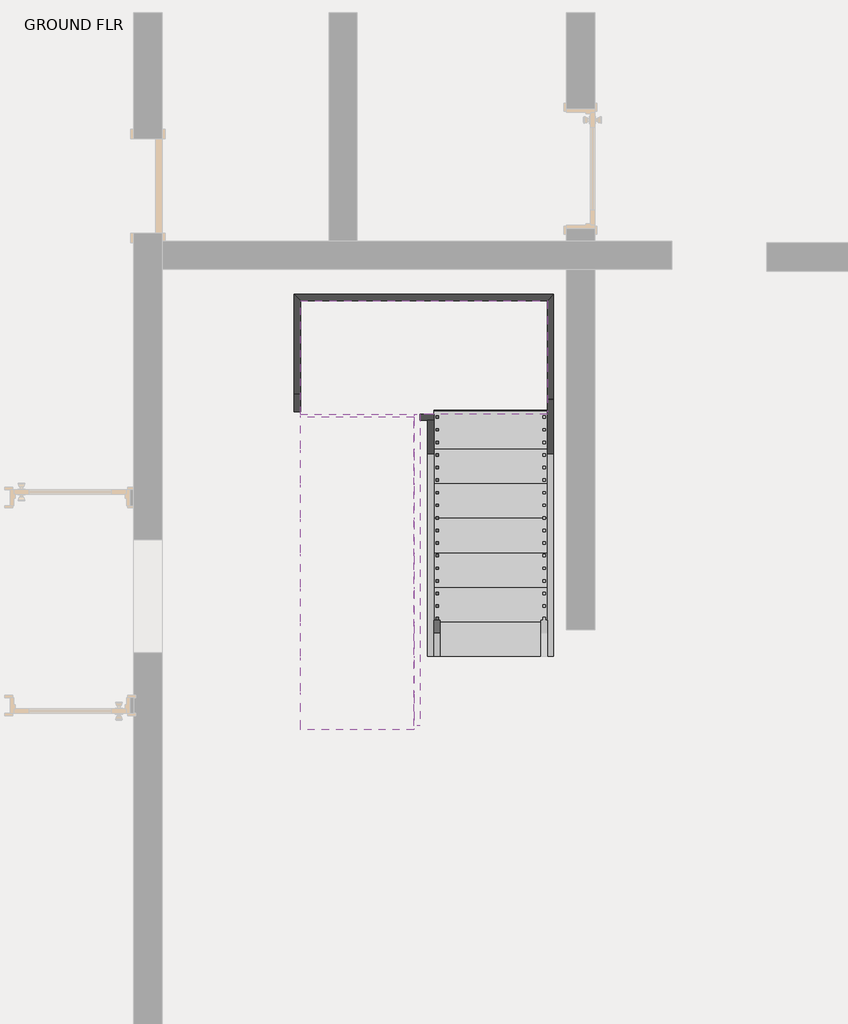
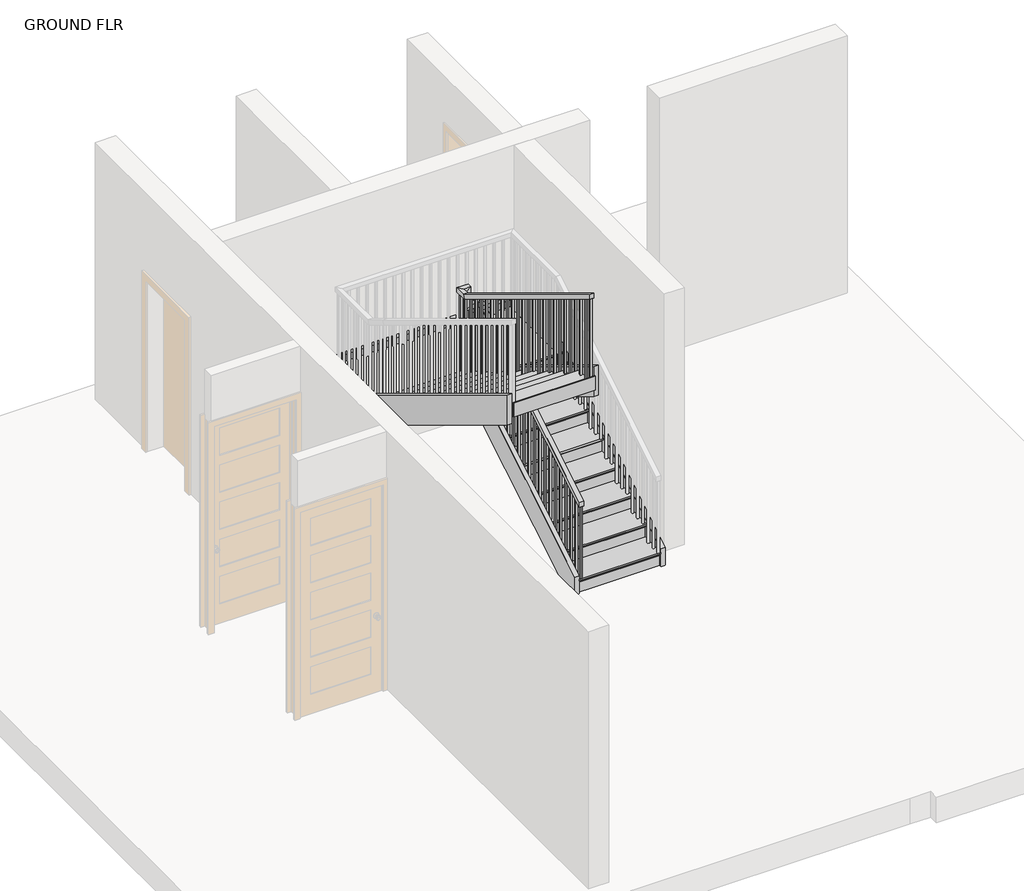
# One storey, part 3 of 3: 8 members, 2 stair flights, 1 railing, 1 slab.
"""IFC4 building model written with IfcOpenShell, lengths in millimetres."""

from ifc_helpers import new_model, si_unit, frame, origin, place, context, project, spatial, polyline, outline, extrude, faceted_brep, transform, mapped, element, save
from components import non_monolithic_landing_8dc99a10, stair_flight_27979845, stair_flight_611140c6

model = new_model("IFC4")

# Units and contexts
model_context = context("Model", 3, world=origin())
ifc_project = project(units=[si_unit("LENGTHUNIT", "METRE", prefix="MILLI")], contexts=[model_context])

# Site, building, storey
site = spatial("IfcSite", under=ifc_project)
building = spatial("IfcBuilding", under=site)
storey = spatial("IfcBuildingStorey", under=building, Name="GROUND FLR", Elevation=609.6)

# Members
placement = place(None, origin())
element("IfcMember", 1, ObjectType="Stringer - 2\" Width", at=placement, inside=storey, context=model_context, shape_type="SweptSolid", body=[
    extrude(outline(polyline([(-3250.5249317, 609.6), (-3250.5249317, 821.714512), (-1345.5249317, 1976.2599665), (-1345.5249317, 1619.851205), (-3012.4394199, 609.6), (-3250.5249317, 609.6)])), frame((-6345.6481169, 0.0, 0.0), z_axis=(1.0, 0.0, 0.0), x_axis=(0.0, 1.0, 0.0)), (0.0, 0.0, 1.0), 50.8),
])
element("IfcMember", 2, ObjectType="Stringer - 2\" Width", at=placement, inside=storey, context=model_context, shape_type="SweptSolid", body=[
    extrude(outline(polyline([(-3250.5249317, 609.6), (-3250.5249317, 821.714512), (-1239.5838764, 2040.4666667), (-1154.4294199, 1735.6666667), (-3012.4394199, 609.6), (-3250.5249317, 609.6)])), frame((-5380.4481169, 0.0, 0.0), z_axis=(1.0, 0.0, 0.0), x_axis=(0.0, 1.0, 0.0)), (0.0, 0.0, 1.0), 50.8),
])
element("IfcMember", 3, ObjectType="Stringer - 2\" Width", at=placement, inside=storey, context=model_context, shape_type="SweptSolid", body=[
    extrude(outline(polyline([(-1294.7249317, 2176.3811786), (-1294.7249317, 1819.9724171), (-3809.3249317, 3343.9724171), (-3809.3249317, 3700.3811786), (-1294.7249317, 2176.3811786)])), frame((-6457.6431792, 0.0, 0.0), z_axis=(1.0, 0.0, 0.0), x_axis=(0.0, 1.0, 0.0)), (0.0, 0.0, 1.0), 50.8),
])
element("IfcMember", 4, ObjectType="Stringer - 2\" Width", at=placement, inside=storey, context=model_context, shape_type="SweptSolid", body=[
    extrude(outline(polyline([(-1070.465987, 2040.4666667), (-1155.6204435, 1735.6666667), (-3809.3249317, 3343.9724171), (-3809.3249317, 3700.3811786), (-1070.465987, 2040.4666667)])), frame((-7422.8431792, 0.0, 0.0), z_axis=(1.0, 0.0, 0.0), x_axis=(0.0, 1.0, 0.0)), (0.0, 0.0, 1.0), 50.8),
])
element("IfcMember", 5, ObjectType="Stringer - 2\" Width", at=placement, inside=storey, context=model_context, shape_type="SweptSolid", body=[
    extrude(outline(polyline([(-6406.8431792, -1345.5249317), (-6406.8431792, -1294.7249317), (-6294.8481169, -1294.7249317), (-6294.8481169, -1345.5249317), (-6406.8431792, -1345.5249317)])), frame((0.0, 0.0, 1735.6666667), z_axis=(0.0, 0.0, 1.0), x_axis=(1.0, 0.0, 0.0)), (0.0, 0.0, 1.0), 304.8),
])
element("IfcMember", 6, ObjectType="Stringer - 2\" Width", at=placement, inside=storey, context=model_context, shape_type="Brep", body=[
    faceted_brep([(-5380.4481169, -1239.5838764, 2040.4666667), (-5329.6481169, -1239.5838764, 2040.4666667), (-5329.6481169, -329.5249317, 2040.4666667), (-5380.4481169, -380.3249317, 2040.4666667), (-5380.4481169, -1154.4294199, 1735.6666667), (-5380.4481169, -380.3249317, 1735.6666667), (-5329.6481169, -1154.4294199, 1735.6666667), (-5329.6481169, -329.5249317, 1735.6666667)], [[[0, 1, 2, 3]], [[4, 0, 3, 5]], [[6, 4, 5, 7]], [[1, 6, 7, 2]], [[1, 0, 4, 6]], [[2, 7, 5, 3]]]),
])
element("IfcMember", 7, ObjectType="Stringer - 2\" Width", at=placement, inside=storey, context=model_context, shape_type="SweptSolid", body=[
    extrude(outline(polyline([(-5329.6481169, -329.5249317), (-5380.4481169, -380.3249317), (-7372.0431792, -380.3249317), (-7422.8431792, -329.5249317), (-5329.6481169, -329.5249317)])), frame((0.0, 0.0, 1735.6666667), z_axis=(0.0, 0.0, 1.0), x_axis=(1.0, 0.0, 0.0)), (0.0, 0.0, 1.0), 304.8),
])
element("IfcMember", 8, ObjectType="Stringer - 2\" Width", at=placement, inside=storey, context=model_context, shape_type="Brep", body=[
    faceted_brep([(-7372.0431792, -380.3249317, 2040.4666667), (-7422.8431792, -329.5249317, 2040.4666667), (-7422.8431792, -1070.465987, 2040.4666667), (-7372.0431792, -1070.465987, 2040.4666667), (-7372.0431792, -380.3249317, 1735.6666667), (-7372.0431792, -1155.6204435, 1735.6666667), (-7422.8431792, -329.5249317, 1735.6666667), (-7422.8431792, -1155.6204435, 1735.6666667)], [[[0, 1, 2, 3]], [[4, 0, 3, 5]], [[6, 4, 5, 7]], [[1, 6, 7, 2]], [[1, 0, 4, 6]], [[2, 7, 5, 3]]]),
])

# Railing
element("IfcRailing", 9, ObjectType="Handrail - Rectangular", at=placement, inside=storey, context=model_context, shape_type="SolidModel", body=[
    faceted_brep([(-6294.8481169, -3250.5249317, 1693.3333333), (-6294.8481169, -3250.5249317, 1633.9318731), (-6244.0481169, -3250.5249317, 1633.9318731), (-6244.0481169, -3250.5249317, 1693.3333333), (-6294.8481169, -1370.9249317, 2832.4848485), (-6294.8481169, -1320.1249317, 2803.871267), (-6244.0481169, -1320.1249317, 2803.871267), (-6244.0481169, -1370.9249317, 2832.4848485), (-6294.8481169, -1370.9249317, 2878.6666667), (-6294.8481169, -1320.1249317, 2827.8666667), (-6244.0481169, -1320.1249317, 2827.8666667), (-6244.0481169, -1370.9249317, 2878.6666667), (-6294.8481169, -1294.7249317, 2878.6666667), (-6294.8481169, -1294.7249317, 2827.8666667), (-6244.0481169, -1243.9249317, 2827.8666667), (-6244.0481169, -1243.9249317, 2878.6666667), (-6371.0481169, -1294.7249317, 2878.6666667), (-6371.0481169, -1294.7249317, 2827.8666667), (-6371.0481169, -1243.9249317, 2827.8666667), (-6371.0481169, -1243.9249317, 2878.6666667), (-6381.4431792, -1294.7249317, 2878.6666667), (-6432.2431792, -1294.7249317, 2827.8666667), (-6432.2431792, -1243.9249317, 2827.8666667), (-6381.4431792, -1243.9249317, 2878.6666667), (-6381.4431792, -1294.7249317, 3094.1818182), (-6432.2431792, -1294.7249317, 3043.3818182), (-6432.2431792, -1243.9249317, 3043.3818182), (-6381.4431792, -1243.9249317, 3094.1818182), (-6457.6431792, -1294.7249317, 3094.1818182), (-6457.6431792, -1294.7249317, 3043.3818182), (-6508.4431792, -1243.9249317, 3043.3818182), (-6508.4431792, -1243.9249317, 3094.1818182), (-6457.6431792, -1370.9249317, 3094.1818182), (-6457.6431792, -1385.1173411, 3043.3818182), (-6508.4431792, -1385.1173411, 3043.3818182), (-6508.4431792, -1370.9249317, 3094.1818182), (-6457.6431792, -3809.3249317, 4572.0), (-6508.4431792, -3809.3249317, 4572.0), (-6508.4431792, -3809.3249317, 4512.5985397), (-6457.6431792, -3809.3249317, 4512.5985397)], [[[0, 1, 2, 3]], [[1, 0, 4, 5]], [[2, 1, 5, 6]], [[3, 2, 6, 7]], [[0, 3, 7, 4]], [[5, 4, 8, 9]], [[6, 5, 9, 10]], [[7, 6, 10, 11]], [[4, 7, 11, 8]], [[9, 8, 12, 13]], [[10, 9, 13, 14]], [[11, 10, 14, 15]], [[8, 11, 15, 12]], [[13, 12, 16, 17]], [[14, 13, 17, 18]], [[15, 14, 18, 19]], [[12, 15, 19, 16]], [[17, 16, 20, 21]], [[18, 17, 21, 22]], [[19, 18, 22, 23]], [[16, 19, 23, 20]], [[21, 20, 24, 25]], [[22, 21, 25, 26]], [[23, 22, 26, 27]], [[20, 23, 27, 24]], [[25, 24, 28, 29]], [[26, 25, 29, 30]], [[27, 26, 30, 31]], [[24, 27, 31, 28]], [[29, 28, 32, 33]], [[30, 29, 33, 34]], [[31, 30, 34, 35]], [[28, 31, 35, 32]], [[36, 37, 38, 39]], [[33, 32, 36, 39]], [[34, 33, 39, 38]], [[35, 34, 38, 37]], [[32, 35, 37, 36]]]),
    extrude(outline(polyline([(-3698.1999317, 4445.2500549), (-3698.1999317, 3488.2666667), (-3717.2499317, 3488.2666667), (-3717.2499317, 4456.7955094), (-3698.1999317, 4445.2500549)])), frame((-6492.5681792, 0.0, 0.0), z_axis=(1.0, 0.0, 0.0), x_axis=(0.0, 1.0, 0.0)), (0.0, 0.0, 1.0), 19.05),
    extrude(outline(polyline([(-3596.5999317, 4383.6742973), (-3596.5999317, 3488.2666667), (-3615.6499317, 3488.2666667), (-3615.6499317, 4395.2197519), (-3596.5999317, 4383.6742973)])), frame((-6492.5681792, 0.0, 0.0), z_axis=(1.0, 0.0, 0.0), x_axis=(0.0, 1.0, 0.0)), (0.0, 0.0, 1.0), 19.05),
    extrude(outline(polyline([(-3494.9999317, 4322.0985397), (-3494.9999317, 3318.9333333), (-3514.0499317, 3318.9333333), (-3514.0499317, 4333.6439943), (-3494.9999317, 4322.0985397)])), frame((-6492.5681792, 0.0, 0.0), z_axis=(1.0, 0.0, 0.0), x_axis=(0.0, 1.0, 0.0)), (0.0, 0.0, 1.0), 19.05),
    extrude(outline(polyline([(-3393.3999317, 4260.5227822), (-3393.3999317, 3318.9333333), (-3412.4499317, 3318.9333333), (-3412.4499317, 4272.0682367), (-3393.3999317, 4260.5227822)])), frame((-6492.5681792, 0.0, 0.0), z_axis=(1.0, 0.0, 0.0), x_axis=(0.0, 1.0, 0.0)), (0.0, 0.0, 1.0), 19.05),
    extrude(outline(polyline([(-3291.7999317, 4198.9470246), (-3291.7999317, 3318.9333333), (-3310.8499317, 3318.9333333), (-3310.8499317, 4210.4924791), (-3291.7999317, 4198.9470246)])), frame((-6492.5681792, 0.0, 0.0), z_axis=(1.0, 0.0, 0.0), x_axis=(0.0, 1.0, 0.0)), (0.0, 0.0, 1.0), 19.05),
    extrude(outline(polyline([(-3190.1999317, 4137.371267), (-3190.1999317, 3149.6), (-3209.2499317, 3149.6), (-3209.2499317, 4148.9167216), (-3190.1999317, 4137.371267)])), frame((-6492.5681792, 0.0, 0.0), z_axis=(1.0, 0.0, 0.0), x_axis=(0.0, 1.0, 0.0)), (0.0, 0.0, 1.0), 19.05),
    extrude(outline(polyline([(-3088.5999317, 4075.7955094), (-3088.5999317, 3149.6), (-3107.6499317, 3149.6), (-3107.6499317, 4087.340964), (-3088.5999317, 4075.7955094)])), frame((-6492.5681792, 0.0, 0.0), z_axis=(1.0, 0.0, 0.0), x_axis=(0.0, 1.0, 0.0)), (0.0, 0.0, 1.0), 19.05),
    extrude(outline(polyline([(-2986.9999317, 4014.2197519), (-2986.9999317, 3149.6), (-3006.0499317, 3149.6), (-3006.0499317, 4025.7652064), (-2986.9999317, 4014.2197519)])), frame((-6492.5681792, 0.0, 0.0), z_axis=(1.0, 0.0, 0.0), x_axis=(0.0, 1.0, 0.0)), (0.0, 0.0, 1.0), 19.05),
    extrude(outline(polyline([(-2885.3999317, 3952.6439943), (-2885.3999317, 2980.2666667), (-2904.4499317, 2980.2666667), (-2904.4499317, 3964.1894488), (-2885.3999317, 3952.6439943)])), frame((-6492.5681792, 0.0, 0.0), z_axis=(1.0, 0.0, 0.0), x_axis=(0.0, 1.0, 0.0)), (0.0, 0.0, 1.0), 19.05),
    extrude(outline(polyline([(-2783.7999317, 3891.0682367), (-2783.7999317, 2980.2666667), (-2802.8499317, 2980.2666667), (-2802.8499317, 3902.6136913), (-2783.7999317, 3891.0682367)])), frame((-6492.5681792, 0.0, 0.0), z_axis=(1.0, 0.0, 0.0), x_axis=(0.0, 1.0, 0.0)), (0.0, 0.0, 1.0), 19.05),
    extrude(outline(polyline([(-2682.1999317, 3829.4924791), (-2682.1999317, 2980.2666667), (-2701.2499317, 2980.2666667), (-2701.2499317, 3841.0379337), (-2682.1999317, 3829.4924791)])), frame((-6492.5681792, 0.0, 0.0), z_axis=(1.0, 0.0, 0.0), x_axis=(0.0, 1.0, 0.0)), (0.0, 0.0, 1.0), 19.05),
    extrude(outline(polyline([(-2580.5999317, 3767.9167216), (-2580.5999317, 2810.9333333), (-2599.6499317, 2810.9333333), (-2599.6499317, 3779.4621761), (-2580.5999317, 3767.9167216)])), frame((-6492.5681792, 0.0, 0.0), z_axis=(1.0, 0.0, 0.0), x_axis=(0.0, 1.0, 0.0)), (0.0, 0.0, 1.0), 19.05),
    extrude(outline(polyline([(-2478.9999317, 3706.340964), (-2478.9999317, 2810.9333333), (-2498.0499317, 2810.9333333), (-2498.0499317, 3717.8864185), (-2478.9999317, 3706.340964)])), frame((-6492.5681792, 0.0, 0.0), z_axis=(1.0, 0.0, 0.0), x_axis=(0.0, 1.0, 0.0)), (0.0, 0.0, 1.0), 19.05),
    extrude(outline(polyline([(-2377.3999317, 3644.7652064), (-2377.3999317, 2641.6), (-2396.4499317, 2641.6), (-2396.4499317, 3656.310661), (-2377.3999317, 3644.7652064)])), frame((-6492.5681792, 0.0, 0.0), z_axis=(1.0, 0.0, 0.0), x_axis=(0.0, 1.0, 0.0)), (0.0, 0.0, 1.0), 19.05),
    extrude(outline(polyline([(-2275.7999317, 3583.1894488), (-2275.7999317, 2641.6), (-2294.8499317, 2641.6), (-2294.8499317, 3594.7349034), (-2275.7999317, 3583.1894488)])), frame((-6492.5681792, 0.0, 0.0), z_axis=(1.0, 0.0, 0.0), x_axis=(0.0, 1.0, 0.0)), (0.0, 0.0, 1.0), 19.05),
    extrude(outline(polyline([(-2174.1999317, 3521.6136913), (-2174.1999317, 2641.6), (-2193.2499317, 2641.6), (-2193.2499317, 3533.1591458), (-2174.1999317, 3521.6136913)])), frame((-6492.5681792, 0.0, 0.0), z_axis=(1.0, 0.0, 0.0), x_axis=(0.0, 1.0, 0.0)), (0.0, 0.0, 1.0), 19.05),
    extrude(outline(polyline([(-2072.5999317, 3460.0379337), (-2072.5999317, 2472.2666667), (-2091.6499317, 2472.2666667), (-2091.6499317, 3471.5833882), (-2072.5999317, 3460.0379337)])), frame((-6492.5681792, 0.0, 0.0), z_axis=(1.0, 0.0, 0.0), x_axis=(0.0, 1.0, 0.0)), (0.0, 0.0, 1.0), 19.05),
    extrude(outline(polyline([(-1970.9999317, 3398.4621761), (-1970.9999317, 2472.2666667), (-1990.0499317, 2472.2666667), (-1990.0499317, 3410.0076307), (-1970.9999317, 3398.4621761)])), frame((-6492.5681792, 0.0, 0.0), z_axis=(1.0, 0.0, 0.0), x_axis=(0.0, 1.0, 0.0)), (0.0, 0.0, 1.0), 19.05),
    extrude(outline(polyline([(-1869.3999317, 3336.8864185), (-1869.3999317, 2472.2666667), (-1888.4499317, 2472.2666667), (-1888.4499317, 3348.4318731), (-1869.3999317, 3336.8864185)])), frame((-6492.5681792, 0.0, 0.0), z_axis=(1.0, 0.0, 0.0), x_axis=(0.0, 1.0, 0.0)), (0.0, 0.0, 1.0), 19.05),
    extrude(outline(polyline([(-1767.7999317, 3275.310661), (-1767.7999317, 2302.9333333), (-1786.8499317, 2302.9333333), (-1786.8499317, 3286.8561155), (-1767.7999317, 3275.310661)])), frame((-6492.5681792, 0.0, 0.0), z_axis=(1.0, 0.0, 0.0), x_axis=(0.0, 1.0, 0.0)), (0.0, 0.0, 1.0), 19.05),
    extrude(outline(polyline([(-1666.1999317, 3213.7349034), (-1666.1999317, 2302.9333333), (-1685.2499317, 2302.9333333), (-1685.2499317, 3225.2803579), (-1666.1999317, 3213.7349034)])), frame((-6492.5681792, 0.0, 0.0), z_axis=(1.0, 0.0, 0.0), x_axis=(0.0, 1.0, 0.0)), (0.0, 0.0, 1.0), 19.05),
    extrude(outline(polyline([(-1564.5999317, 3152.1591458), (-1564.5999317, 2302.9333333), (-1583.6499317, 2302.9333333), (-1583.6499317, 3163.7046004), (-1564.5999317, 3152.1591458)])), frame((-6492.5681792, 0.0, 0.0), z_axis=(1.0, 0.0, 0.0), x_axis=(0.0, 1.0, 0.0)), (0.0, 0.0, 1.0), 19.05),
    extrude(outline(polyline([(-1462.9999317, 3090.5833882), (-1462.9999317, 2133.6), (-1482.0499317, 2133.6), (-1482.0499317, 3102.1288428), (-1462.9999317, 3090.5833882)])), frame((-6492.5681792, 0.0, 0.0), z_axis=(1.0, 0.0, 0.0), x_axis=(0.0, 1.0, 0.0)), (0.0, 0.0, 1.0), 19.05),
    extrude(outline(polyline([(-1361.3999317, 3029.0076307), (-1361.3999317, 2133.6), (-1380.4499317, 2133.6), (-1380.4499317, 3040.5530852), (-1361.3999317, 3029.0076307)])), frame((-6492.5681792, 0.0, 0.0), z_axis=(1.0, 0.0, 0.0), x_axis=(0.0, 1.0, 0.0)), (0.0, 0.0, 1.0), 19.05),
    extrude(outline(polyline([(-6463.1231169, -1278.8499317), (-6482.1731169, -1278.8499317), (-6482.1731169, -1259.7999317), (-6463.1231169, -1259.7999317), (-6463.1231169, -1278.8499317)])), frame((0.0, 0.0, 1964.2666667), z_axis=(0.0, 0.0, 1.0), x_axis=(1.0, 0.0, 0.0)), (0.0, 0.0, 1.0), 1079.1151515),
    extrude(outline(polyline([(-6361.5231169, -1278.8499317), (-6380.5731169, -1278.8499317), (-6380.5731169, -1259.7999317), (-6361.5231169, -1259.7999317), (-6361.5231169, -1278.8499317)])), frame((0.0, 0.0, 1964.2666667), z_axis=(0.0, 0.0, 1.0), x_axis=(1.0, 0.0, 0.0)), (0.0, 0.0, 1.0), 863.6),
    extrude(outline(polyline([(-6278.9731169, -1329.6499317), (-6278.9731169, -1310.5999317), (-6259.9231169, -1310.5999317), (-6259.9231169, -1329.6499317), (-6278.9731169, -1329.6499317)])), frame((0.0, 0.0, 1794.9333333), z_axis=(0.0, 0.0, 1.0), x_axis=(1.0, 0.0, 0.0)), (0.0, 0.0, 1.0), 1032.9333333),
    extrude(outline(polyline([(-1412.1999317, 2748.0682367), (-1412.1999317, 1794.9333333), (-1431.2499317, 1794.9333333), (-1431.2499317, 2736.5227822), (-1412.1999317, 2748.0682367)])), frame((-6278.9731169, 0.0, 0.0), z_axis=(1.0, 0.0, 0.0), x_axis=(0.0, 1.0, 0.0)), (0.0, 0.0, 1.0), 19.05),
    extrude(outline(polyline([(-1513.7999317, 2686.4924791), (-1513.7999317, 1794.9333333), (-1532.8499317, 1794.9333333), (-1532.8499317, 2674.9470246), (-1513.7999317, 2686.4924791)])), frame((-6278.9731169, 0.0, 0.0), z_axis=(1.0, 0.0, 0.0), x_axis=(0.0, 1.0, 0.0)), (0.0, 0.0, 1.0), 19.05),
    extrude(outline(polyline([(-1615.3999317, 2624.9167216), (-1615.3999317, 1625.6), (-1634.4499317, 1625.6), (-1634.4499317, 2613.371267), (-1615.3999317, 2624.9167216)])), frame((-6278.9731169, 0.0, 0.0), z_axis=(1.0, 0.0, 0.0), x_axis=(0.0, 1.0, 0.0)), (0.0, 0.0, 1.0), 19.05),
    extrude(outline(polyline([(-1716.9999317, 2563.340964), (-1716.9999317, 1625.6), (-1736.0499317, 1625.6), (-1736.0499317, 2551.7955094), (-1716.9999317, 2563.340964)])), frame((-6278.9731169, 0.0, 0.0), z_axis=(1.0, 0.0, 0.0), x_axis=(0.0, 1.0, 0.0)), (0.0, 0.0, 1.0), 19.05),
    extrude(outline(polyline([(-1818.5999317, 2501.7652064), (-1818.5999317, 1625.6), (-1837.6499317, 1625.6), (-1837.6499317, 2490.2197519), (-1818.5999317, 2501.7652064)])), frame((-6278.9731169, 0.0, 0.0), z_axis=(1.0, 0.0, 0.0), x_axis=(0.0, 1.0, 0.0)), (0.0, 0.0, 1.0), 19.05),
    extrude(outline(polyline([(-1920.1999317, 2440.1894488), (-1920.1999317, 1456.2666667), (-1939.2499317, 1456.2666667), (-1939.2499317, 2428.6439943), (-1920.1999317, 2440.1894488)])), frame((-6278.9731169, 0.0, 0.0), z_axis=(1.0, 0.0, 0.0), x_axis=(0.0, 1.0, 0.0)), (0.0, 0.0, 1.0), 19.05),
    extrude(outline(polyline([(-2021.7999317, 2378.6136913), (-2021.7999317, 1456.2666667), (-2040.8499317, 1456.2666667), (-2040.8499317, 2367.0682367), (-2021.7999317, 2378.6136913)])), frame((-6278.9731169, 0.0, 0.0), z_axis=(1.0, 0.0, 0.0), x_axis=(0.0, 1.0, 0.0)), (0.0, 0.0, 1.0), 19.05),
    extrude(outline(polyline([(-2123.3999317, 2317.0379337), (-2123.3999317, 1456.2666667), (-2142.4499317, 1456.2666667), (-2142.4499317, 2305.4924791), (-2123.3999317, 2317.0379337)])), frame((-6278.9731169, 0.0, 0.0), z_axis=(1.0, 0.0, 0.0), x_axis=(0.0, 1.0, 0.0)), (0.0, 0.0, 1.0), 19.05),
    extrude(outline(polyline([(-2224.9999317, 2255.4621761), (-2224.9999317, 1286.9333333), (-2244.0499317, 1286.9333333), (-2244.0499317, 2243.9167216), (-2224.9999317, 2255.4621761)])), frame((-6278.9731169, 0.0, 0.0), z_axis=(1.0, 0.0, 0.0), x_axis=(0.0, 1.0, 0.0)), (0.0, 0.0, 1.0), 19.05),
    extrude(outline(polyline([(-2326.5999317, 2193.8864185), (-2326.5999317, 1286.9333333), (-2345.6499317, 1286.9333333), (-2345.6499317, 2182.340964), (-2326.5999317, 2193.8864185)])), frame((-6278.9731169, 0.0, 0.0), z_axis=(1.0, 0.0, 0.0), x_axis=(0.0, 1.0, 0.0)), (0.0, 0.0, 1.0), 19.05),
    extrude(outline(polyline([(-2428.1999317, 2132.310661), (-2428.1999317, 1117.6), (-2447.2499317, 1117.6), (-2447.2499317, 2120.7652064), (-2428.1999317, 2132.310661)])), frame((-6278.9731169, 0.0, 0.0), z_axis=(1.0, 0.0, 0.0), x_axis=(0.0, 1.0, 0.0)), (0.0, 0.0, 1.0), 19.05),
    extrude(outline(polyline([(-2529.7999317, 2070.7349034), (-2529.7999317, 1117.6), (-2548.8499317, 1117.6), (-2548.8499317, 2059.1894488), (-2529.7999317, 2070.7349034)])), frame((-6278.9731169, 0.0, 0.0), z_axis=(1.0, 0.0, 0.0), x_axis=(0.0, 1.0, 0.0)), (0.0, 0.0, 1.0), 19.05),
    extrude(outline(polyline([(-2631.3999317, 2009.1591458), (-2631.3999317, 1117.6), (-2650.4499317, 1117.6), (-2650.4499317, 1997.6136913), (-2631.3999317, 2009.1591458)])), frame((-6278.9731169, 0.0, 0.0), z_axis=(1.0, 0.0, 0.0), x_axis=(0.0, 1.0, 0.0)), (0.0, 0.0, 1.0), 19.05),
    extrude(outline(polyline([(-2732.9999317, 1947.5833882), (-2732.9999317, 948.2666667), (-2752.0499317, 948.2666667), (-2752.0499317, 1936.0379337), (-2732.9999317, 1947.5833882)])), frame((-6278.9731169, 0.0, 0.0), z_axis=(1.0, 0.0, 0.0), x_axis=(0.0, 1.0, 0.0)), (0.0, 0.0, 1.0), 19.05),
    extrude(outline(polyline([(-2834.5999317, 1886.0076307), (-2834.5999317, 948.2666667), (-2853.6499317, 948.2666667), (-2853.6499317, 1874.4621761), (-2834.5999317, 1886.0076307)])), frame((-6278.9731169, 0.0, 0.0), z_axis=(1.0, 0.0, 0.0), x_axis=(0.0, 1.0, 0.0)), (0.0, 0.0, 1.0), 19.05),
    extrude(outline(polyline([(-2936.1999317, 1824.4318731), (-2936.1999317, 948.2666667), (-2955.2499317, 948.2666667), (-2955.2499317, 1812.8864185), (-2936.1999317, 1824.4318731)])), frame((-6278.9731169, 0.0, 0.0), z_axis=(1.0, 0.0, 0.0), x_axis=(0.0, 1.0, 0.0)), (0.0, 0.0, 1.0), 19.05),
    extrude(outline(polyline([(-3037.7999317, 1762.8561155), (-3037.7999317, 778.9333333), (-3056.8499317, 778.9333333), (-3056.8499317, 1751.310661), (-3037.7999317, 1762.8561155)])), frame((-6278.9731169, 0.0, 0.0), z_axis=(1.0, 0.0, 0.0), x_axis=(0.0, 1.0, 0.0)), (0.0, 0.0, 1.0), 19.05),
    extrude(outline(polyline([(-3139.3999317, 1701.2803579), (-3139.3999317, 778.9333333), (-3158.4499317, 778.9333333), (-3158.4499317, 1689.7349034), (-3139.3999317, 1701.2803579)])), frame((-6278.9731169, 0.0, 0.0), z_axis=(1.0, 0.0, 0.0), x_axis=(0.0, 1.0, 0.0)), (0.0, 0.0, 1.0), 19.05),
    extrude(outline(polyline([(-6473.5181792, -1278.8499317), (-6492.5681792, -1278.8499317), (-6492.5681792, -1259.7999317), (-6473.5181792, -1259.7999317), (-6473.5181792, -1278.8499317)])), frame((0.0, 0.0, 1964.2666667), z_axis=(0.0, 0.0, 1.0), x_axis=(1.0, 0.0, 0.0)), (0.0, 0.0, 1.0), 1079.1151515),
    extrude(outline(polyline([(-6278.9731169, -1278.8499317), (-6278.9731169, -1259.7999317), (-6259.9231169, -1259.7999317), (-6259.9231169, -1278.8499317), (-6278.9731169, -1278.8499317)])), frame((0.0, 0.0, 1964.2666667), z_axis=(0.0, 0.0, 1.0), x_axis=(1.0, 0.0, 0.0)), (0.0, 0.0, 1.0), 863.6),
    extrude(outline(polyline([(-3790.2749317, 4501.0530852), (-3790.2749317, 3488.2666667), (-3809.3249317, 3488.2666667), (-3809.3249317, 4512.5985397), (-3790.2749317, 4501.0530852)])), frame((-6492.5681792, 0.0, 0.0), z_axis=(1.0, 0.0, 0.0), x_axis=(0.0, 1.0, 0.0)), (0.0, 0.0, 1.0), 19.05),
    extrude(outline(polyline([(-3231.4749317, 1645.4773276), (-3231.4749317, 778.9333333), (-3250.5249317, 778.9333333), (-3250.5249317, 1633.9318731), (-3231.4749317, 1645.4773276)])), frame((-6278.9731169, 0.0, 0.0), z_axis=(1.0, 0.0, 0.0), x_axis=(0.0, 1.0, 0.0)), (0.0, 0.0, 1.0), 19.05),
])

# Slab
non_monolithic_landing_shape = non_monolithic_landing_8dc99a10(model_context)
element("IfcSlab", 10, ObjectType="Non-Monolithic Landing", at=placement, inside=storey, context=model_context, shape_type="MappedRepresentation", body=[
    mapped(non_monolithic_landing_shape, transform((0.0, 0.0, 0.0), x_axis=(1.0, 0.0, 0.0), y_axis=(0.0, 1.0, 0.0), z_axis=(0.0, 0.0, 1.0))),
])

# Stair flights
stair_flight_shape = stair_flight_27979845(model_context)
element("IfcStairFlight", 11, ObjectType="2\" Tread 1\" Nosing 1/4\" Riser", at=placement, inside=storey, context=model_context, shape_type="MappedRepresentation", body=[
    mapped(stair_flight_shape, transform((0.0, 0.0, 0.0), x_axis=(1.0, 0.0, 0.0), y_axis=(0.0, 1.0, 0.0), z_axis=(0.0, 0.0, 1.0))),
])
stair_flight_2_shape = stair_flight_611140c6(model_context)
element("IfcStairFlight", 12, ObjectType="2\" Tread 1\" Nosing 1/4\" Riser", at=placement, inside=storey, context=model_context, shape_type="MappedRepresentation", body=[
    mapped(stair_flight_2_shape, transform((0.0, 0.0, 0.0), x_axis=(1.0, 0.0, 0.0), y_axis=(0.0, 1.0, 0.0), z_axis=(0.0, 0.0, 1.0))),
])

save(model, "model.ifc")

# Revit data of these elements
# Type "Handrail - Rectangular"
#   Assembly Code = "C2010400"
#   built-in parameter 1008612 = 0.0416667 (stored number, unit not read)
#   built-in parameter 1008611 = 0.0416667 (stored number, unit not read)
#   built-in parameter 1008609 = 0.333333 (stored number, unit not read)
#   built-in parameter 1008604 = 0.166667 (stored number, unit not read)
#   built-in parameter 1008603 = 0.166667 (stored number, unit not read)
#   Railing Height = 3' - 0"
#   built-in parameter 1008630 = 2
#   built-in parameter 1008610 = 2
#   built-in parameter 1008618 = Baluster - Square : 3/4"
# Elements 1, 2, 3, 4, 5, 6, 7, 8 (IfcMember, "Stringer - 2\" Width")
#   Phase Created = New Construction
# Element 9 (IfcRailing, "Handrail - Rectangular")
#   Phase Created = New Construction
# Element 10 (IfcSlab, "Non-Monolithic Landing")
#   Phase Created = New Construction
# Elements 11, 12 (IfcStairFlight, "2\" Tread 1\" Nosing 1/4\" Riser")
#   Phase Created = New Construction
